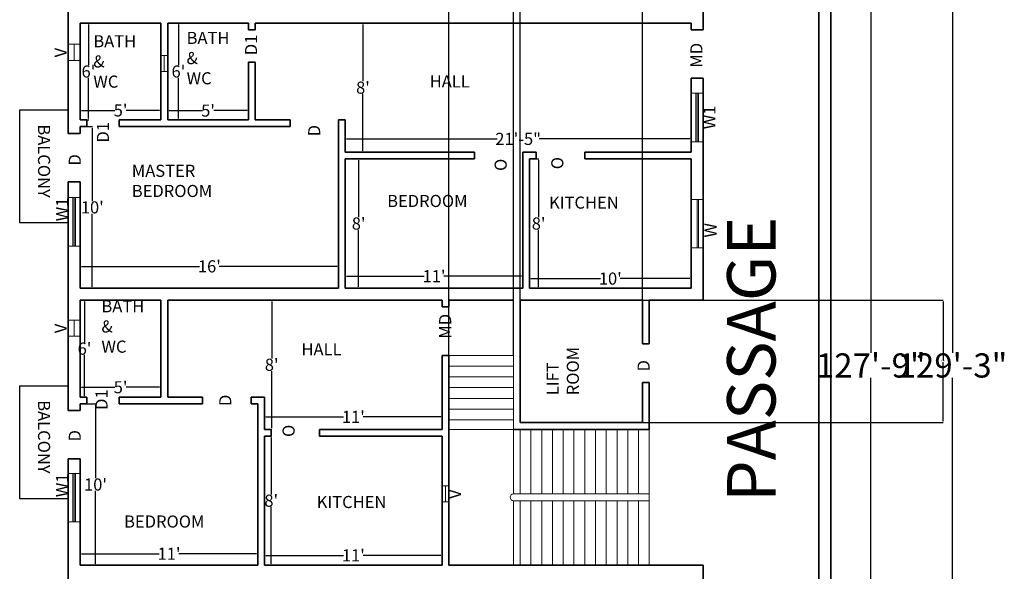
# Model space of a CAD drawing. Units: inches. Extents: x -2189 to 546, y 945 to 2684.
# Tile 3 of 10: x -866 to -134, y 1672 to 2082. Entities that reach past the tile are written whole.
import ezdxf

# ---------------------------------------------------------------- set-up
doc = ezdxf.new("R2010")
doc.units = ezdxf.units.IN
doc.header["$MEASUREMENT"] = 0
for name, color, linetype, lineweight in [('A-ANNO-DIMS', 2, 'Continuous', 13), ('A-ANNO-TEXT', 7, 'Continuous', 18), ('A-AREA-IDEN', 3, 'Continuous', 18), ('A-FLOR-BALC', 8, 'Continuous', 25), ('A-FLOR-STRS', 3, 'Continuous', 18), ('A-GLAZ', 4, 'Continuous', 18), ('A-WALL', 7, 'Continuous', 35)]:
    doc.layers.add(name, color=color, linetype=linetype, lineweight=lineweight)
doc.styles.get("Standard").update_dxf_attribs({"font": 'arial.ttf'})
doc.dimstyles.get("Standard").update_dxf_attribs({"dimtxt": 1, "dimasz": 1, "dimexe": 0.18, "dimexo": 0.0625, "dimgap": 0.09, "dimtad": 0, "dimtih": 1, "dimtoh": 1, "dimdec": 0, "dimzin": 0, "dimdsep": 46, "dimlunit": 3, "dimtxsty": 'Standard', "dimcen": 0.09, "dimadec": 0, "dimazin": 0, "dimtfac": 1, "dimtdec": 0, "dimtofl": 0, "dimtmove": 0, "dimatfit": 3, "dimfxl": 1, "dimtolj": 1, "dimtzin": 0, "dimarcsym": 0})

# ---------------------------------------------------------------- blocks, each defined once
blk = doc.blocks.new('*D37')
at = {"layer": 'A-ANNO-DIMS', "color": 0, "lineweight": -2, "transparency": 16777216}
for p, q in [((-820.78, 1676.24), (-820.78, 1684.89)), ((-819.78, 1684.71), (-762.08, 1684.71)), ((-689.78, 1684.71), (-747.48, 1684.71)), ((-688.78, 1676.24), (-688.78, 1684.89))]:
    blk.add_line(p, q, dxfattribs=at)
at = {"layer": 'A-ANNO-DIMS', "color": 0, "transparency": 16777216}
for points in [[(-819.78, 1684.88), (-819.78, 1684.54), (-820.78, 1684.71)], [(-689.78, 1684.88), (-689.78, 1684.54), (-688.78, 1684.71)]]:
    blk.add_solid(points, dxfattribs=at)
at = {"layer": 'Defpoints', "color": 0, "transparency": 16777216}
for p in [(-688.78, 1684.71), (-820.78, 1676.17), (-688.78, 1676.17)]:
    blk.add_point(p, dxfattribs=at)
at = {"layer": 'A-ANNO-DIMS', "color": 0, "transparency": 16777216, "insert": (-754.78, 1684.71), "char_height": 1, "attachment_point": 5}
blk.add_mtext("\\A1;{\\H9x;11'}", dxfattribs=at)
blk = doc.blocks.new('*D38')
at = {"layer": 'A-ANNO-DIMS', "color": 0, "lineweight": -2, "transparency": 16777216}
for p, q in [((-820.72, 1796.17), (-809.26, 1796.17)), ((-809.44, 1795.17), (-809.44, 1740.86)), ((-809.44, 1677.17), (-809.44, 1731.49)), ((-820.72, 1676.17), (-809.26, 1676.17))]:
    blk.add_line(p, q, dxfattribs=at)
at = {"layer": 'A-ANNO-DIMS', "color": 0, "transparency": 16777216}
for points in [[(-809.61, 1795.17), (-809.28, 1795.17), (-809.44, 1796.17)], [(-809.61, 1677.17), (-809.28, 1677.17), (-809.44, 1676.17)]]:
    blk.add_solid(points, dxfattribs=at)
at = {"layer": 'Defpoints', "color": 0, "transparency": 16777216}
for p in [(-820.78, 1796.17), (-809.44, 1796.17), (-820.78, 1676.17)]:
    blk.add_point(p, dxfattribs=at)
at = {"layer": 'A-ANNO-DIMS', "color": 0, "transparency": 16777216, "insert": (-809.44, 1736.17), "char_height": 1, "attachment_point": 5}
blk.add_mtext("\\A1;{\\H9x;10'}", dxfattribs=at)
blk = doc.blocks.new('*D39')
at = {"layer": 'A-ANNO-DIMS', "color": 0, "lineweight": -2, "transparency": 16777216}
for p, q in [((-820.78, 1801.24), (-820.78, 1808.68)), ((-819.78, 1808.5), (-795.01, 1808.5)), ((-761.78, 1808.5), (-786.55, 1808.5)), ((-760.78, 1801.24), (-760.78, 1808.68))]:
    blk.add_line(p, q, dxfattribs=at)
at = {"layer": 'A-ANNO-DIMS', "color": 0, "transparency": 16777216}
for points in [[(-819.78, 1808.66), (-819.78, 1808.33), (-820.78, 1808.5)], [(-761.78, 1808.66), (-761.78, 1808.33), (-760.78, 1808.5)]]:
    blk.add_solid(points, dxfattribs=at)
at = {"layer": 'Defpoints', "color": 0, "transparency": 16777216}
for p in [(-760.78, 1808.5), (-820.78, 1801.17), (-760.78, 1801.17)]:
    blk.add_point(p, dxfattribs=at)
at = {"layer": 'A-ANNO-DIMS', "color": 0, "transparency": 16777216, "insert": (-790.78, 1808.5), "char_height": 1, "attachment_point": 5}
blk.add_mtext("\\A1;{\\H9x;5'}", dxfattribs=at)
blk = doc.blocks.new('*D40')
at = {"layer": 'A-ANNO-DIMS', "color": 0, "lineweight": -2, "transparency": 16777216}
for p, q in [((-820.72, 1873.17), (-817.43, 1873.17)), ((-817.61, 1872.17), (-817.61, 1841.86)), ((-817.61, 1802.17), (-817.61, 1832.49)), ((-820.72, 1801.17), (-817.43, 1801.17))]:
    blk.add_line(p, q, dxfattribs=at)
at = {"layer": 'A-ANNO-DIMS', "color": 0, "transparency": 16777216}
for points in [[(-817.77, 1872.17), (-817.44, 1872.17), (-817.61, 1873.17)], [(-817.77, 1802.17), (-817.44, 1802.17), (-817.61, 1801.17)]]:
    blk.add_solid(points, dxfattribs=at)
at = {"layer": 'Defpoints', "color": 0, "transparency": 16777216}
for p in [(-820.78, 1873.17), (-817.61, 1873.17), (-820.78, 1801.17)]:
    blk.add_point(p, dxfattribs=at)
at = {"layer": 'A-ANNO-DIMS', "color": 0, "transparency": 16777216, "insert": (-817.61, 1837.17), "char_height": 1, "attachment_point": 5}
blk.add_mtext("\\A1;{\\H9x;6'}", dxfattribs=at)
blk = doc.blocks.new('*D41')
at = {"layer": 'A-ANNO-DIMS', "color": 0, "lineweight": -2, "transparency": 16777216}
for p, q in [((-683.78, 1676.24), (-683.78, 1683.7)), ((-682.78, 1683.52), (-625.08, 1683.52)), ((-552.78, 1683.52), (-610.48, 1683.52)), ((-551.78, 1676.24), (-551.78, 1683.7))]:
    blk.add_line(p, q, dxfattribs=at)
at = {"layer": 'A-ANNO-DIMS', "color": 0, "transparency": 16777216}
for points in [[(-682.78, 1683.68), (-682.78, 1683.35), (-683.78, 1683.52)], [(-552.78, 1683.68), (-552.78, 1683.35), (-551.78, 1683.52)]]:
    blk.add_solid(points, dxfattribs=at)
at = {"layer": 'Defpoints', "color": 0, "transparency": 16777216}
for p in [(-551.78, 1683.52), (-683.78, 1676.17), (-551.78, 1676.17)]:
    blk.add_point(p, dxfattribs=at)
at = {"layer": 'A-ANNO-DIMS', "color": 0, "transparency": 16777216, "insert": (-617.78, 1683.52), "char_height": 1, "attachment_point": 5}
blk.add_mtext("\\A1;{\\H9x;11'}", dxfattribs=at)
blk = doc.blocks.new('*D42')
at = {"layer": 'A-ANNO-DIMS', "color": 0, "lineweight": -2, "transparency": 16777216}
for p, q in [((-683.72, 1772.17), (-678.62, 1772.17)), ((-678.8, 1771.17), (-678.8, 1728.86)), ((-678.8, 1677.17), (-678.8, 1719.49)), ((-683.72, 1676.17), (-678.62, 1676.17))]:
    blk.add_line(p, q, dxfattribs=at)
at = {"layer": 'A-ANNO-DIMS', "color": 0, "transparency": 16777216}
for points in [[(-678.97, 1771.17), (-678.63, 1771.17), (-678.8, 1772.17)], [(-678.97, 1677.17), (-678.63, 1677.17), (-678.8, 1676.17)]]:
    blk.add_solid(points, dxfattribs=at)
at = {"layer": 'Defpoints', "color": 0, "transparency": 16777216}
for p in [(-683.78, 1772.17), (-683.78, 1676.17), (-678.8, 1676.17)]:
    blk.add_point(p, dxfattribs=at)
at = {"layer": 'A-ANNO-DIMS', "color": 0, "transparency": 16777216, "insert": (-678.8, 1724.17), "char_height": 1, "attachment_point": 5}
blk.add_mtext("\\A1;{\\H9x;8'}", dxfattribs=at)
blk = doc.blocks.new('*D43')
at = {"layer": 'A-ANNO-DIMS', "color": 0, "lineweight": -2, "transparency": 16777216}
for p, q in [((-683.72, 1873.17), (-678.29, 1873.17)), ((-678.47, 1872.17), (-678.47, 1829.86)), ((-678.47, 1778.17), (-678.47, 1820.49)), ((-683.72, 1777.17), (-678.29, 1777.17))]:
    blk.add_line(p, q, dxfattribs=at)
at = {"layer": 'A-ANNO-DIMS', "color": 0, "transparency": 16777216}
for points in [[(-678.64, 1872.17), (-678.31, 1872.17), (-678.47, 1873.17)], [(-678.64, 1778.17), (-678.31, 1778.17), (-678.47, 1777.17)]]:
    blk.add_solid(points, dxfattribs=at)
at = {"layer": 'Defpoints', "color": 0, "transparency": 16777216}
for p in [(-683.78, 1873.17), (-678.47, 1873.17), (-683.78, 1777.17)]:
    blk.add_point(p, dxfattribs=at)
at = {"layer": 'A-ANNO-DIMS', "color": 0, "transparency": 16777216, "insert": (-678.47, 1825.17), "char_height": 1, "attachment_point": 5}
blk.add_mtext("\\A1;{\\H9x;8'}", dxfattribs=at)
blk = doc.blocks.new('*D44')
at = {"layer": 'A-ANNO-DIMS', "color": 0, "lineweight": -2, "transparency": 16777216}
for p, q in [((-683.78, 1777.24), (-683.78, 1786.65)), ((-682.78, 1786.47), (-625.08, 1786.47)), ((-552.78, 1786.47), (-610.48, 1786.47)), ((-551.78, 1777.24), (-551.78, 1786.65))]:
    blk.add_line(p, q, dxfattribs=at)
at = {"layer": 'A-ANNO-DIMS', "color": 0, "transparency": 16777216}
for points in [[(-682.78, 1786.64), (-682.78, 1786.31), (-683.78, 1786.47)], [(-552.78, 1786.64), (-552.78, 1786.31), (-551.78, 1786.47)]]:
    blk.add_solid(points, dxfattribs=at)
at = {"layer": 'Defpoints', "color": 0, "transparency": 16777216}
for p in [(-551.78, 1786.47), (-683.78, 1777.17), (-551.78, 1777.17)]:
    blk.add_point(p, dxfattribs=at)
at = {"layer": 'A-ANNO-DIMS', "color": 0, "transparency": 16777216, "insert": (-617.78, 1786.47), "char_height": 1, "attachment_point": 5}
blk.add_mtext("\\A1;{\\H9x;11'}", dxfattribs=at)
blk = doc.blocks.new('*D45')
at = {"layer": 'A-ANNO-DIMS', "color": 0, "lineweight": -2, "transparency": 16777216}
for p, q in [((-820.78, 1882.24), (-820.78, 1898.51)), ((-819.78, 1898.33), (-732.08, 1898.33)), ((-629.78, 1898.33), (-717.48, 1898.33)), ((-628.78, 1882.24), (-628.78, 1898.51))]:
    blk.add_line(p, q, dxfattribs=at)
at = {"layer": 'A-ANNO-DIMS', "color": 0, "transparency": 16777216}
for points in [[(-819.78, 1898.5), (-819.78, 1898.16), (-820.78, 1898.33)], [(-629.78, 1898.5), (-629.78, 1898.16), (-628.78, 1898.33)]]:
    blk.add_solid(points, dxfattribs=at)
at = {"layer": 'Defpoints', "color": 0, "transparency": 16777216}
for p in [(-628.78, 1898.33), (-820.78, 1882.17), (-628.78, 1882.17)]:
    blk.add_point(p, dxfattribs=at)
at = {"layer": 'A-ANNO-DIMS', "color": 0, "transparency": 16777216, "insert": (-724.78, 1898.33), "char_height": 1, "attachment_point": 5}
blk.add_mtext("\\A1;{\\H9x;16'}", dxfattribs=at)
blk = doc.blocks.new('*D46')
at = {"layer": 'A-ANNO-DIMS', "color": 0, "lineweight": -2, "transparency": 16777216}
for p, q in [((-820.72, 2002.17), (-811.63, 2002.17)), ((-811.81, 2001.17), (-811.81, 1946.86)), ((-811.81, 1883.17), (-811.81, 1937.49)), ((-820.72, 1882.17), (-811.63, 1882.17))]:
    blk.add_line(p, q, dxfattribs=at)
at = {"layer": 'A-ANNO-DIMS', "color": 0, "transparency": 16777216}
for points in [[(-811.98, 2001.17), (-811.65, 2001.17), (-811.81, 2002.17)], [(-811.98, 1883.17), (-811.65, 1883.17), (-811.81, 1882.17)]]:
    blk.add_solid(points, dxfattribs=at)
at = {"layer": 'Defpoints', "color": 0, "transparency": 16777216}
for p in [(-820.78, 2002.17), (-820.78, 1882.17), (-811.81, 1882.17)]:
    blk.add_point(p, dxfattribs=at)
at = {"layer": 'A-ANNO-DIMS', "color": 0, "transparency": 16777216, "insert": (-811.81, 1942.17), "char_height": 1, "attachment_point": 5}
blk.add_mtext("\\A1;{\\H9x;10'}", dxfattribs=at)
blk = doc.blocks.new('*D47')
at = {"layer": 'A-ANNO-DIMS', "color": 0, "lineweight": -2, "transparency": 16777216}
for p, q in [((-820.78, 2007.24), (-820.78, 2014.43)), ((-819.78, 2014.25), (-795.01, 2014.25)), ((-761.78, 2014.25), (-786.55, 2014.25)), ((-760.78, 2007.24), (-760.78, 2014.43))]:
    blk.add_line(p, q, dxfattribs=at)
at = {"layer": 'A-ANNO-DIMS', "color": 0, "transparency": 16777216}
for points in [[(-819.78, 2014.42), (-819.78, 2014.08), (-820.78, 2014.25)], [(-761.78, 2014.42), (-761.78, 2014.08), (-760.78, 2014.25)]]:
    blk.add_solid(points, dxfattribs=at)
at = {"layer": 'Defpoints', "color": 0, "transparency": 16777216}
for p in [(-760.78, 2014.25), (-820.78, 2007.17), (-760.78, 2007.17)]:
    blk.add_point(p, dxfattribs=at)
at = {"layer": 'A-ANNO-DIMS', "color": 0, "transparency": 16777216, "insert": (-790.78, 2014.25), "char_height": 1, "attachment_point": 5}
blk.add_mtext("\\A1;{\\H9x;5'}", dxfattribs=at)
blk = doc.blocks.new('*D48')
at = {"layer": 'A-ANNO-DIMS', "color": 0, "lineweight": -2, "transparency": 16777216}
for p, q in [((-820.72, 2079.17), (-814.5, 2079.17)), ((-814.68, 2078.17), (-814.68, 2047.86)), ((-814.68, 2008.17), (-814.68, 2038.49)), ((-820.72, 2007.17), (-814.5, 2007.17))]:
    blk.add_line(p, q, dxfattribs=at)
at = {"layer": 'A-ANNO-DIMS', "color": 0, "transparency": 16777216}
for points in [[(-814.84, 2078.17), (-814.51, 2078.17), (-814.68, 2079.17)], [(-814.84, 2008.17), (-814.51, 2008.17), (-814.68, 2007.17)]]:
    blk.add_solid(points, dxfattribs=at)
at = {"layer": 'Defpoints', "color": 0, "transparency": 16777216}
for p in [(-820.78, 2079.17), (-814.68, 2079.17), (-820.78, 2007.17)]:
    blk.add_point(p, dxfattribs=at)
at = {"layer": 'A-ANNO-DIMS', "color": 0, "transparency": 16777216, "insert": (-814.68, 2043.17), "char_height": 1, "attachment_point": 5}
blk.add_mtext("\\A1;{\\H9x;6'}", dxfattribs=at)
blk = doc.blocks.new('*D49')
at = {"layer": 'A-ANNO-DIMS', "color": 0, "lineweight": -2, "transparency": 16777216}
for p, q in [((-755.78, 2007.24), (-755.78, 2014.31)), ((-754.78, 2014.13), (-730.01, 2014.13)), ((-696.78, 2014.13), (-721.55, 2014.13)), ((-695.78, 2007.24), (-695.78, 2014.31))]:
    blk.add_line(p, q, dxfattribs=at)
at = {"layer": 'A-ANNO-DIMS', "color": 0, "transparency": 16777216}
for points in [[(-754.78, 2014.3), (-754.78, 2013.96), (-755.78, 2014.13)], [(-696.78, 2014.3), (-696.78, 2013.96), (-695.78, 2014.13)]]:
    blk.add_solid(points, dxfattribs=at)
at = {"layer": 'Defpoints', "color": 0, "transparency": 16777216}
for p in [(-755.78, 2014.13), (-755.78, 2007.17), (-695.78, 2007.17)]:
    blk.add_point(p, dxfattribs=at)
at = {"layer": 'A-ANNO-DIMS', "color": 0, "transparency": 16777216, "insert": (-725.78, 2014.13), "char_height": 1, "attachment_point": 5}
blk.add_mtext("\\A1;{\\H9x;5'}", dxfattribs=at)
blk = doc.blocks.new('*D50')
at = {"layer": 'A-ANNO-DIMS', "color": 0, "lineweight": -2, "transparency": 16777216}
for p, q in [((-755.72, 2079.17), (-747.61, 2079.17)), ((-747.79, 2078.17), (-747.79, 2047.86)), ((-747.79, 2008.17), (-747.79, 2038.49)), ((-755.72, 2007.17), (-747.61, 2007.17))]:
    blk.add_line(p, q, dxfattribs=at)
at = {"layer": 'A-ANNO-DIMS', "color": 0, "transparency": 16777216}
for points in [[(-747.95, 2078.17), (-747.62, 2078.17), (-747.79, 2079.17)], [(-747.95, 2008.17), (-747.62, 2008.17), (-747.79, 2007.17)]]:
    blk.add_solid(points, dxfattribs=at)
at = {"layer": 'Defpoints', "color": 0, "transparency": 16777216}
for p in [(-755.78, 2079.17), (-747.79, 2079.17), (-755.78, 2007.17)]:
    blk.add_point(p, dxfattribs=at)
at = {"layer": 'A-ANNO-DIMS', "color": 0, "transparency": 16777216, "insert": (-747.79, 2043.17), "char_height": 1, "attachment_point": 5}
blk.add_mtext("\\A1;{\\H9x;6'}", dxfattribs=at)
blk = doc.blocks.new('*D51')
at = {"layer": 'A-ANNO-DIMS', "color": 0, "lineweight": -2, "transparency": 16777216}
for p, q in [((-623.78, 1882.24), (-623.78, 1891.19)), ((-622.78, 1891.01), (-565.08, 1891.01)), ((-492.78, 1891.01), (-550.48, 1891.01)), ((-491.78, 1882.24), (-491.78, 1891.19))]:
    blk.add_line(p, q, dxfattribs=at)
at = {"layer": 'A-ANNO-DIMS', "color": 0, "transparency": 16777216}
for points in [[(-622.78, 1891.17), (-622.78, 1890.84), (-623.78, 1891.01)], [(-492.78, 1891.17), (-492.78, 1890.84), (-491.78, 1891.01)]]:
    blk.add_solid(points, dxfattribs=at)
at = {"layer": 'Defpoints', "color": 0, "transparency": 16777216}
for p in [(-623.78, 1891.01), (-623.78, 1882.17), (-491.78, 1882.17)]:
    blk.add_point(p, dxfattribs=at)
at = {"layer": 'A-ANNO-DIMS', "color": 0, "transparency": 16777216, "insert": (-557.78, 1891.01), "char_height": 1, "attachment_point": 5}
blk.add_mtext("\\A1;{\\H9x;11'}", dxfattribs=at)
blk = doc.blocks.new('*D52')
at = {"layer": 'A-ANNO-DIMS', "color": 0, "lineweight": -2, "transparency": 16777216}
for p, q in [((-623.72, 1978.17), (-613.65, 1978.17)), ((-613.83, 1977.17), (-613.83, 1934.86)), ((-613.83, 1883.17), (-613.83, 1925.49)), ((-623.72, 1882.17), (-613.65, 1882.17))]:
    blk.add_line(p, q, dxfattribs=at)
at = {"layer": 'A-ANNO-DIMS', "color": 0, "transparency": 16777216}
for points in [[(-613.99, 1977.17), (-613.66, 1977.17), (-613.83, 1978.17)], [(-613.99, 1883.17), (-613.66, 1883.17), (-613.83, 1882.17)]]:
    blk.add_solid(points, dxfattribs=at)
at = {"layer": 'Defpoints', "color": 0, "transparency": 16777216}
for p in [(-623.78, 1978.17), (-613.83, 1978.17), (-623.78, 1882.17)]:
    blk.add_point(p, dxfattribs=at)
at = {"layer": 'A-ANNO-DIMS', "color": 0, "transparency": 16777216, "insert": (-613.83, 1930.17), "char_height": 1, "attachment_point": 5}
blk.add_mtext("\\A1;{\\H9x;8'}", dxfattribs=at)
blk = doc.blocks.new('*D53')
at = {"layer": 'A-ANNO-DIMS', "color": 0, "lineweight": -2, "transparency": 16777216}
for p, q in [((-486.72, 1978.17), (-479.88, 1978.17)), ((-480.06, 1977.17), (-480.06, 1934.86)), ((-480.06, 1883.17), (-480.06, 1925.49)), ((-486.72, 1882.17), (-479.88, 1882.17))]:
    blk.add_line(p, q, dxfattribs=at)
at = {"layer": 'A-ANNO-DIMS', "color": 0, "transparency": 16777216}
for points in [[(-480.23, 1977.17), (-479.9, 1977.17), (-480.06, 1978.17)], [(-480.23, 1883.17), (-479.9, 1883.17), (-480.06, 1882.17)]]:
    blk.add_solid(points, dxfattribs=at)
at = {"layer": 'Defpoints', "color": 0, "transparency": 16777216}
for p in [(-486.78, 1978.17), (-480.06, 1978.17), (-486.78, 1882.17)]:
    blk.add_point(p, dxfattribs=at)
at = {"layer": 'A-ANNO-DIMS', "color": 0, "transparency": 16777216, "insert": (-480.06, 1930.17), "char_height": 1, "attachment_point": 5}
blk.add_mtext("\\A1;{\\H9x;8'}", dxfattribs=at)
blk = doc.blocks.new('*D54')
at = {"layer": 'A-ANNO-DIMS', "color": 0, "lineweight": -2, "transparency": 16777216}
for p, q in [((-486.78, 1882.24), (-486.78, 1889.42)), ((-485.78, 1889.24), (-434.08, 1889.24)), ((-367.78, 1889.24), (-419.48, 1889.24)), ((-366.78, 1882.24), (-366.78, 1889.42))]:
    blk.add_line(p, q, dxfattribs=at)
at = {"layer": 'A-ANNO-DIMS', "color": 0, "transparency": 16777216}
for points in [[(-485.78, 1889.4), (-485.78, 1889.07), (-486.78, 1889.24)], [(-367.78, 1889.4), (-367.78, 1889.07), (-366.78, 1889.24)]]:
    blk.add_solid(points, dxfattribs=at)
at = {"layer": 'Defpoints', "color": 0, "transparency": 16777216}
for p in [(-486.78, 1889.24), (-486.78, 1882.17), (-366.78, 1882.17)]:
    blk.add_point(p, dxfattribs=at)
at = {"layer": 'A-ANNO-DIMS', "color": 0, "transparency": 16777216, "insert": (-426.78, 1889.24), "char_height": 1, "attachment_point": 5}
blk.add_mtext("\\A1;{\\H9x;10'}", dxfattribs=at)
blk = doc.blocks.new('*D55')
at = {"layer": 'A-ANNO-DIMS', "color": 0, "lineweight": -2, "transparency": 16777216}
for p, q in [((-623.72, 2079.17), (-610.46, 2079.17)), ((-610.64, 2078.17), (-610.64, 2035.86)), ((-610.64, 1984.17), (-610.64, 2026.49)), ((-623.72, 1983.17), (-610.46, 1983.17))]:
    blk.add_line(p, q, dxfattribs=at)
at = {"layer": 'A-ANNO-DIMS', "color": 0, "transparency": 16777216}
for points in [[(-610.81, 2078.17), (-610.48, 2078.17), (-610.64, 2079.17)], [(-610.81, 1984.17), (-610.48, 1984.17), (-610.64, 1983.17)]]:
    blk.add_solid(points, dxfattribs=at)
at = {"layer": 'Defpoints', "color": 0, "transparency": 16777216}
for p in [(-623.78, 2079.17), (-610.64, 2079.17), (-623.78, 1983.17)]:
    blk.add_point(p, dxfattribs=at)
at = {"layer": 'A-ANNO-DIMS', "color": 0, "transparency": 16777216, "insert": (-610.64, 2031.17), "char_height": 1, "attachment_point": 5}
blk.add_mtext("\\A1;{\\H9x;8'}", dxfattribs=at)
blk = doc.blocks.new('*D56')
at = {"layer": 'A-ANNO-DIMS', "color": 0, "lineweight": -2, "transparency": 16777216}
for p, q in [((-623.78, 1983.24), (-623.78, 1993.26)), ((-622.78, 1993.08), (-510.9, 1993.08)), ((-367.78, 1993.08), (-479.65, 1993.08)), ((-366.78, 1983.24), (-366.78, 1993.26))]:
    blk.add_line(p, q, dxfattribs=at)
at = {"layer": 'A-ANNO-DIMS', "color": 0, "transparency": 16777216}
for points in [[(-622.78, 1993.24), (-622.78, 1992.91), (-623.78, 1993.08)], [(-367.78, 1993.24), (-367.78, 1992.91), (-366.78, 1993.08)]]:
    blk.add_solid(points, dxfattribs=at)
at = {"layer": 'Defpoints', "color": 0, "transparency": 16777216}
for p in [(-623.78, 1993.08), (-623.78, 1983.17), (-366.78, 1983.17)]:
    blk.add_point(p, dxfattribs=at)
at = {"layer": 'A-ANNO-DIMS', "color": 0, "transparency": 16777216, "insert": (-495.28, 1993.08), "char_height": 1, "attachment_point": 5}
blk.add_mtext('\\A1;{\\H9x;21\'-5"}', dxfattribs=at)
blk = doc.blocks.new('*D79')
at = {"layer": 'A-ANNO-DIMS', "color": 0, "lineweight": -2, "transparency": 16777216}
for p, q in [((-262.72, 2600.17), (-172.26, 2600.17)), ((-172.44, 2599.17), (-172.44, 1833.96)), ((-172.44, 1050.17), (-172.44, 1815.39)), ((-262.72, 1049.17), (-172.26, 1049.17))]:
    blk.add_line(p, q, dxfattribs=at)
at = {"layer": 'A-ANNO-DIMS', "color": 0, "transparency": 16777216}
for points in [[(-172.6, 2599.17), (-172.27, 2599.17), (-172.44, 2600.17)], [(-172.6, 1050.17), (-172.27, 1050.17), (-172.44, 1049.17)]]:
    blk.add_solid(points, dxfattribs=at)
at = {"layer": 'Defpoints', "color": 0, "transparency": 16777216}
for p in [(-262.78, 2600.17), (-172.44, 2600.17), (-262.78, 1049.17)]:
    blk.add_point(p, dxfattribs=at)
at = {"layer": 'A-ANNO-DIMS', "color": 0, "transparency": 16777216, "insert": (-172.44, 1824.67), "char_height": 1, "attachment_point": 5}
blk.add_mtext('\\A1;{\\H18x;129\'-3"}', dxfattribs=at)
blk = doc.blocks.new('*D80')
at = {"layer": 'A-ANNO-DIMS', "color": 0, "lineweight": -2, "transparency": 16777216}
for p, q in [((-271.72, 2591.17), (-233.01, 2591.17)), ((-233.19, 2590.17), (-233.19, 1833.95)), ((-233.19, 1059.17), (-233.19, 1815.39)), ((-271.72, 1058.17), (-233.01, 1058.17))]:
    blk.add_line(p, q, dxfattribs=at)
at = {"layer": 'A-ANNO-DIMS', "color": 0, "transparency": 16777216}
for points in [[(-233.36, 2590.17), (-233.03, 2590.17), (-233.19, 2591.17)], [(-233.36, 1059.17), (-233.03, 1059.17), (-233.19, 1058.17)]]:
    blk.add_solid(points, dxfattribs=at)
at = {"layer": 'Defpoints', "color": 0, "transparency": 16777216}
for p in [(-271.78, 2591.17), (-233.19, 2591.17), (-271.78, 1058.17)]:
    blk.add_point(p, dxfattribs=at)
at = {"layer": 'A-ANNO-DIMS', "color": 0, "transparency": 16777216, "insert": (-233.19, 1824.67), "char_height": 1, "attachment_point": 5}
blk.add_mtext('\\A1;{\\H18x;127\'-9"}', dxfattribs=at)
blk = doc.blocks.new('WIN-36X9')
for p, q in [((0, 5.5), (36, 5.5)), ((0, 5.5), (36, 5.5)), ((0, 4.5), (36, 4.5)), ((0, 3.5), (36, 3.5))]:
    blk.add_line(p, q)
blk.add_lwpolyline([(0, 0), (0, 9), (36, 9), (36, 0)], close=True)
blk = doc.blocks.new('VENT-12X5')
blk.add_line((2.5, 12), (2.5, 0))
blk.add_lwpolyline([(5, 12), (0, 12), (0, 0), (5, 0)], close=True)
blk = doc.blocks.new('WIN-36X9-TWINLINE')
for p, q in [((4.5, 0), (4.5, 36)), ((5.5, 0), (5.5, 36))]:
    blk.add_line(p, q)
blk.add_lwpolyline([(9, 0), (0, 0), (0, 36), (9, 36)], close=True)
blk = doc.blocks.new('VENT-12X9-SINGLELINE')
blk.add_line((4.5, 12), (4.5, 0))
blk.add_lwpolyline([(0, 12), (9, 12), (9, 0), (0, 0)], close=True)
blk = doc.blocks.new('BALCONY-36X84')
for p, q in [((0, 0), (0, 84)), ((0, 84), (36, 84)), ((36, 0), (0, 0))]:
    blk.add_line(p, q)
blk = doc.blocks.new('*D104')
at = {"layer": 'A-ANNO-DIMS', "color": 0, "lineweight": -2, "transparency": 16777216}
for p, q in [((-493.78, 1873.24), (-493.78, 2683.65)), ((-492.78, 2683.47), (-449.69, 2683.47)), ((-403.78, 2683.47), (-446.86, 2683.47)), ((-402.78, 1873.24), (-402.78, 2683.65))]:
    blk.add_line(p, q, dxfattribs=at)
at = {"layer": 'A-ANNO-DIMS', "color": 0, "transparency": 16777216}
for points in [[(-492.78, 2683.64), (-492.78, 2683.31), (-493.78, 2683.47)], [(-403.78, 2683.64), (-403.78, 2683.31), (-402.78, 2683.47)]]:
    blk.add_solid(points, dxfattribs=at)
at = {"layer": 'Defpoints', "color": 0, "transparency": 16777216}
for p in [(-402.78, 2683.47), (-493.78, 1873.17), (-402.78, 1873.17)]:
    blk.add_point(p, dxfattribs=at)
at = {"layer": 'A-ANNO-DIMS', "color": 0, "transparency": 16777216, "insert": (-448.28, 2683.47), "char_height": 1, "attachment_point": 5}
blk.add_mtext('\\A1;7\'-7"', dxfattribs=at)
blk = doc.blocks.new('*D105')
at = {"layer": 'A-ANNO-DIMS', "color": 0, "lineweight": -2, "transparency": 16777216}
for p, q in [((-402.72, 1873.17), (-179.3, 1873.17)), ((-179.48, 1872.17), (-179.48, 1828.26)), ((-179.48, 1783.17), (-179.48, 1827.08)), ((-402.72, 1782.17), (-179.3, 1782.17))]:
    blk.add_line(p, q, dxfattribs=at)
at = {"layer": 'A-ANNO-DIMS', "color": 0, "transparency": 16777216}
for points in [[(-179.65, 1872.17), (-179.31, 1872.17), (-179.48, 1873.17)], [(-179.65, 1783.17), (-179.31, 1783.17), (-179.48, 1782.17)]]:
    blk.add_solid(points, dxfattribs=at)
at = {"layer": 'Defpoints', "color": 0, "transparency": 16777216}
for p in [(-402.78, 1873.17), (-179.48, 1873.17), (-402.78, 1782.17)]:
    blk.add_point(p, dxfattribs=at)
at = {"layer": 'A-ANNO-DIMS', "color": 0, "transparency": 16777216, "insert": (-179.48, 1827.67), "char_height": 1, "attachment_point": 5}
blk.add_mtext('\\A1;7\'-7"', dxfattribs=at)
blk = doc.blocks.new('*D106')
at = {"layer": 'A-ANNO-DIMS', "color": 0, "lineweight": -2, "transparency": 16777216}
for p, q in [((-546.78, 1832.24), (-546.78, 2683.65)), ((-545.78, 2683.47), (-524.22, 2683.47)), ((-499.78, 2683.47), (-521.34, 2683.47)), ((-498.78, 1832.24), (-498.78, 2683.65))]:
    blk.add_line(p, q, dxfattribs=at)
at = {"layer": 'A-ANNO-DIMS', "color": 0, "transparency": 16777216}
for points in [[(-545.78, 2683.64), (-545.78, 2683.31), (-546.78, 2683.47)], [(-499.78, 2683.64), (-499.78, 2683.31), (-498.78, 2683.47)]]:
    blk.add_solid(points, dxfattribs=at)
at = {"layer": 'Defpoints', "color": 0, "transparency": 16777216}
for p in [(-498.78, 2683.47), (-546.78, 1832.17), (-498.78, 1832.17)]:
    blk.add_point(p, dxfattribs=at)
at = {"layer": 'A-ANNO-DIMS', "color": 0, "transparency": 16777216, "insert": (-522.78, 2683.47), "char_height": 1, "attachment_point": 5}
blk.add_mtext('\\A1;4\'-0"', dxfattribs=at)

msp = doc.modelspace()

# ---------------------------------------------------------------- linework, layer by layer
at = {"layer": 'A-FLOR-STRS'}
for p, q in [((-498.78, 1729.17), (-498.78, 1873.17)), ((-546.78, 1832.17), (-498.78, 1832.17)), ((-546.78, 1824.17), (-498.78, 1824.17)), ((-546.78, 1816.17), (-498.78, 1816.17)), ((-546.78, 1808.17), (-498.78, 1808.17)), ((-546.78, 1800.17), (-498.78, 1800.17)), ((-546.78, 1792.17), (-498.78, 1792.17)), ((-546.78, 1792.17), (-498.78, 1792.17)), ((-546.78, 1784.17), (-498.78, 1784.17)), ((-546.78, 1777.17), (-498.78, 1777.17)), ((-493.78, 1729.17), (-493.78, 1777.16)), ((-485.78, 1729.17), (-485.78, 1777.16)), ((-477.78, 1729.17), (-477.78, 1777.16)), ((-469.78, 1729.17), (-469.78, 1777.16)), ((-461.78, 1729.17), (-461.78, 1777.16)), ((-453.78, 1729.17), (-453.78, 1777.16)), ((-445.78, 1729.17), (-445.78, 1777.16)), ((-437.78, 1729.17), (-437.78, 1777.16)), ((-429.78, 1729.17), (-429.78, 1777.16)), ((-421.78, 1729.17), (-421.78, 1777.16)), ((-413.78, 1729.17), (-413.78, 1777.16)), ((-405.78, 1729.17), (-405.78, 1777.16)), ((-397.78, 1676.17), (-397.78, 1777.16)), ((-397.78, 1729.17), (-498.78, 1729.17)), ((-498.78, 1676.17), (-498.78, 1724.17)), ((-397.78, 1724.17), (-498.78, 1724.17)), ((-493.78, 1676.17), (-493.78, 1724.17)), ((-485.78, 1676.17), (-485.78, 1724.17)), ((-477.78, 1676.17), (-477.78, 1724.17)), ((-469.78, 1676.17), (-469.78, 1724.17)), ((-461.78, 1676.17), (-461.78, 1724.17)), ((-453.78, 1676.17), (-453.78, 1724.17)), ((-445.78, 1676.17), (-445.78, 1724.17)), ((-437.78, 1676.17), (-437.78, 1724.17)), ((-429.78, 1676.17), (-429.78, 1724.17)), ((-421.78, 1676.17), (-421.78, 1724.17)), ((-413.78, 1676.17), (-413.78, 1724.17)), ((-405.78, 1676.17), (-405.78, 1724.17))]:
    msp.add_line(p, q, dxfattribs=at)
msp.add_arc((-498.78, 1726.67), 2.5, 90, 270, dxfattribs=at)
at = {"layer": 'A-WALL'}
for p, q in [((-262.78, 2600.17), (-262.78, 1049.17)), ((-271.78, 2591.17), (-271.78, 1058.17)), ((-357.78, 2074.17), (-357.78, 2240.2)), ((-829.78, 1997.17), (-829.78, 2163.17)), ((-820.78, 2007.17), (-820.78, 2079.17)), ((-760.78, 2079.17), (-820.78, 2079.17)), ((-760.78, 2007.17), (-760.78, 2079.17)), ((-755.78, 2007.17), (-755.78, 2079.17)), ((-695.78, 2079.17), (-755.78, 2079.17)), ((-695.78, 2074.17), (-695.78, 2079.17)), ((-366.78, 2079.17), (-690.78, 2079.17)), ((-690.78, 2074.17), (-690.78, 2079.17)), ((-366.78, 2074.17), (-366.78, 2079.17)), ((-695.78, 2074.17), (-690.78, 2074.17)), ((-366.78, 2074.17), (-357.78, 2074.17)), ((-695.78, 2007.17), (-695.78, 2050.17)), ((-695.78, 2050.17), (-690.78, 2050.17)), ((-690.78, 2007.17), (-690.78, 2050.17)), ((-366.78, 1983.17), (-366.78, 2038.17)), ((-366.78, 2038.17), (-357.78, 2038.17)), ((-357.78, 1873.17), (-357.78, 2038.17)), ((-815.78, 2007.17), (-820.78, 2007.17)), ((-815.78, 2007.17), (-815.78, 2002.17)), ((-760.78, 2007.17), (-791.78, 2007.17)), ((-791.78, 2007.17), (-791.78, 2002.17)), ((-695.78, 2007.17), (-755.78, 2007.17)), ((-664.78, 2007.17), (-690.78, 2007.17)), ((-664.78, 2002.17), (-664.78, 2007.17)), ((-628.78, 1882.17), (-628.78, 2007.17)), ((-623.78, 2007.17), (-628.78, 2007.17)), ((-623.78, 1983.17), (-623.78, 2007.17)), ((-820.78, 1997.17), (-820.78, 2002.17)), ((-815.78, 2002.17), (-820.78, 2002.17)), ((-664.78, 2002.17), (-791.78, 2002.17)), ((-820.78, 1997.17), (-829.78, 1997.17)), ((-527.78, 1983.17), (-623.78, 1983.17)), ((-623.78, 1882.17), (-623.78, 1978.17)), ((-527.78, 1978.17), (-623.78, 1978.17)), ((-527.78, 1983.17), (-527.78, 1978.17)), ((-491.78, 1983.17), (-486.78, 1983.17)), ((-491.78, 1983.17), (-491.78, 1978.17)), ((-491.78, 1882.17), (-491.78, 1978.17)), ((-481.78, 1983.17), (-486.78, 1983.17)), ((-486.78, 1882.17), (-486.78, 1978.17)), ((-481.78, 1978.17), (-486.78, 1978.17)), ((-481.78, 1983.17), (-481.78, 1978.17)), ((-366.78, 1983.17), (-445.78, 1983.17)), ((-445.78, 1983.17), (-445.78, 1978.17)), ((-366.78, 1978.17), (-445.78, 1978.17)), ((-366.78, 1882.17), (-366.78, 1978.17)), ((-829.78, 1791.17), (-829.78, 1961.17)), ((-820.78, 1961.17), (-829.78, 1961.17)), ((-820.78, 1882.17), (-820.78, 1961.17)), ((-628.78, 1882.17), (-820.78, 1882.17)), ((-491.78, 1882.17), (-623.78, 1882.17)), ((-366.78, 1882.17), (-486.78, 1882.17)), ((-820.78, 1801.17), (-820.78, 1873.17)), ((-760.78, 1873.17), (-820.78, 1873.17)), ((-760.78, 1801.17), (-760.78, 1873.17)), ((-755.78, 1801.17), (-755.78, 1873.17)), ((-551.78, 1873.17), (-755.78, 1873.17)), ((-551.78, 1868.17), (-551.78, 1873.17)), ((-551.78, 1868.17), (-546.78, 1868.17)), ((-546.78, 1868.17), (-546.78, 1873.17)), ((-498.78, 1873.17), (-546.78, 1873.17)), ((-493.78, 1782.17), (-493.78, 1873.17)), ((-402.78, 1873.17), (-493.78, 1873.17)), ((-402.78, 1840.74), (-402.78, 1873.17)), ((-357.78, 1873.17), (-397.78, 1873.17)), ((-397.78, 1840.74), (-397.78, 1873.17)), ((-402.78, 1840.74), (-397.78, 1840.74)), ((-551.78, 1777.17), (-551.78, 1832.17)), ((-551.78, 1832.17), (-546.78, 1832.17)), ((-546.78, 1777.17), (-546.78, 1832.17)), ((-402.78, 1782.17), (-402.78, 1811.96)), ((-402.78, 1811.96), (-397.78, 1811.96)), ((-397.78, 1777.16), (-397.78, 1811.96)), ((-815.78, 1801.17), (-820.78, 1801.17)), ((-815.78, 1801.17), (-815.78, 1796.17)), ((-760.78, 1801.17), (-791.78, 1801.17)), ((-791.78, 1801.17), (-791.78, 1796.17)), ((-729.78, 1801.17), (-755.78, 1801.17)), ((-729.78, 1801.17), (-729.78, 1796.17)), ((-683.78, 1801.17), (-693.78, 1801.17)), ((-693.78, 1801.17), (-693.78, 1796.17)), ((-683.78, 1777.17), (-683.78, 1801.17)), ((-820.78, 1791.17), (-820.78, 1796.17)), ((-815.78, 1796.17), (-820.78, 1796.17)), ((-729.78, 1796.17), (-791.78, 1796.17)), ((-688.78, 1796.17), (-693.78, 1796.17)), ((-688.78, 1676.17), (-688.78, 1796.17)), ((-820.78, 1791.17), (-829.78, 1791.17)), ((-402.78, 1782.17), (-493.78, 1782.17)), ((-678.78, 1777.17), (-683.78, 1777.17)), ((-683.78, 1676.17), (-683.78, 1772.17)), ((-678.78, 1772.17), (-683.78, 1772.17)), ((-678.78, 1772.17), (-678.78, 1777.17)), ((-551.78, 1777.17), (-642.84, 1777.17)), ((-642.84, 1772.17), (-642.84, 1777.17)), ((-551.78, 1772.17), (-642.84, 1772.17)), ((-551.78, 1676.17), (-551.78, 1772.17)), ((-546.78, 1772.17), (-546.78, 1777.17)), ((-546.78, 1676.17), (-546.78, 1772.17)), ((-397.78, 1777.17), (-498.78, 1777.17)), ((-829.78, 1585.17), (-829.78, 1755.17)), ((-820.78, 1755.17), (-829.78, 1755.17)), ((-820.78, 1676.17), (-820.78, 1755.17)), ((-688.78, 1676.17), (-820.78, 1676.17)), ((-551.78, 1676.17), (-683.78, 1676.17)), ((-357.78, 1676.17), (-546.78, 1676.17)), ((-357.78, 1662.17), (-357.78, 1676.17))]:
    msp.add_line(p, q, dxfattribs=at)

# ---------------------------------------------------------------- block references
at = {"layer": 'A-FLOR-BALC'}
for p in [(-865.78, 1930.66), (-865.78, 1725.62)]:
    msp.add_blockref('BALCONY-36X84', p, dxfattribs=at)
at = {"layer": 'A-GLAZ'}
for name, p in [('VENT-12X9-SINGLELINE', (-829.78, 2051.41)), ('VENT-12X5', (-760.78, 2043.18)), ('WIN-36X9-TWINLINE', (-366.78, 1912.11)), ('VENT-12X9-SINGLELINE', (-829.78, 1846.37)), ('VENT-12X5', (-551.78, 1723.23))]:
    msp.add_blockref(name, p, dxfattribs=at)
for p, rotation in [((-357.78, 1990.95), 90.00000000000095), ((-820.78, 1913.4), 90.00000000000144), ((-820.78, 1708.36), 90.00000000000205)]:
    msp.add_blockref('WIN-36X9', p, dxfattribs=dict(at, rotation=rotation))

# ---------------------------------------------------------------- texts
at = {"layer": 'A-ANNO-TEXT', "char_height": 9, "attachment_point": 1, "rotation": 90}
for s, width, heights, insert in [('D1', 15.3658, [0], (-698.32, 2055.3)), ('V', 17.5973, [0], (-839.88, 2053.66)), ('MD', 16.482, [0], (-367.28, 2046.05)), ('W1', 11.3125, [0], (-357.59, 2000.22)), ('D1', 15.3658, [0], (-808.38, 1990.33)), ('D', 15.3658, [0], (-651.37, 1994.98)), ('D', 15.3658, [0], (-829.35, 1973.26)), ('O', 18.6541, [0.207], (-512.78, 1969.23)), ('O', 18.6541, [0.207], (-470.67, 1970.5)), ('W1', 11.3125, [0], (-838.78, 1931.83)), ('W', 11.3125, [0], (-356.83, 1919.73)), ('MD', 16.482, [0], (-554.06, 1844.6)), ('V', 17.5973, [0], (-839.88, 1848.63)), ('D', 14.8359, [0], (-406.54, 1820.24)), ('D1', 15.3658, [0], (-809.44, 1791.62)), ('D', 15.3658, [0], (-717.46, 1794.51)), ('O', 18.6541, [0.207], (-670.4, 1771.51)), ('D', 15.3658, [0], (-829.35, 1768.22)), ('W1', 11.3125, [0], (-838.78, 1726.79)), ('V', 17.5973, [0], (-546.78, 1725.45))]:
    msp.add_mtext_dynamic_manual_height_columns(s, width=width, gutter_width=1, heights=heights, dxfattribs=dict(at, insert=insert))
at = {"layer": 'A-AREA-IDEN', "char_height": 9, "attachment_point": 1}
for s, width, heights, insert in [('BATH \\P& \\PWC', 29.3144, [0], (-741.71, 2072.64)), ('BATH \\P& \\PWC', 29.3144, [0], (-811.04, 2070.15)), ('HALL', 37.3459, [0], (-561.01, 2040.29)), ('MASTER BEDROOM', 73.5764, [0], (-782.43, 1973.87)), ('BEDROOM', 73.8205, [0.207], (-592.63, 1951.44)), ('KITCHEN', 69.371, [0], (-472.3, 1950.22)), ('BATH \\P& \\PWC', 29.3144, [0], (-805.01, 1873.17)), ('HALL', 37.3459, [0], (-656.34, 1841.19)), ('KITCHEN', 69.371, [0], (-644.99, 1727.7)), ('BEDROOM', 73.8205, [0.207], (-788.17, 1713.17))]:
    msp.add_mtext_dynamic_manual_height_columns(s, width=width, gutter_width=1, heights=heights, dxfattribs=dict(at, insert=insert))
at = {"layer": 'A-AREA-IDEN', "attachment_point": 1}
for s, width, heights, insert, char_height, rotation in [('BALCONY', 7.0599, [0], (-843.17, 2003.84), 9, 270), ('PASSAGE', 260.6717, [220.33], (-339.98, 1723.09), 36, 90), ('LIFT ROOM', 59.9998, [0], (-474.12, 1802.53), 9, 90), ('BALCONY', 7.0599, [0], (-843.17, 1798.81), 9, 270)]:
    msp.add_mtext_dynamic_manual_height_columns(s, width=width, gutter_width=1, heights=heights, dxfattribs=dict(at, insert=insert, char_height=char_height, rotation=rotation))

# ---------------------------------------------------------------- dimensions: what is measured, and where the dimension line sits
at = {"layer": 'A-ANNO-DIMS'}
for base, p1, p2, picture, middle in [((-498.78, 2683.47), (-546.78, 1832.17), (-498.78, 1832.17), '*D106', (-522.78, 2683.47)), ((-402.78, 2683.47), (-493.78, 1873.17), (-402.78, 1873.17), '*D104', (-448.28, 2683.47))]:
    dim = msp.add_linear_dim(base=base, p1=p1, p2=p2, dimstyle='Standard', override={"dimdec": 1, "dimlfac": 1, "dimrnd": 0, "dimzin": 1, "dimdsep": 46, "dimlunit": 4, "dimfrac": 2}, dxfattribs=at)
    dim.commit()
    dim.dimension.update_dxf_attribs({"geometry": picture, "text_midpoint": middle})
for base, p1, p2, angle, text, picture, middle in [((-172.44, 2600.17), (-262.78, 1049.17), (-262.78, 2600.17), 90, '{\\H18x;<>}', '*D79', (-172.44, 1824.67)), ((-233.19, 2591.17), (-271.78, 1058.17), (-271.78, 2591.17), 90, '{\\H18x;<>}', '*D80', (-233.19, 1824.67)), ((-814.68, 2079.17), (-820.78, 2007.17), (-820.78, 2079.17), 90, '{\\H9x;<>}', '*D48', (-814.68, 2043.17)), ((-747.79, 2079.17), (-755.78, 2007.17), (-755.78, 2079.17), 90, '{\\H9x;<>}', '*D50', (-747.79, 2043.17)), ((-610.64, 2079.17), (-623.78, 1983.17), (-623.78, 2079.17), 90, '{\\H9x;<>}', '*D55', (-610.64, 2031.17)), ((-760.78, 2014.25), (-820.78, 2007.17), (-760.78, 2007.17), 180, '{\\H9x;<>}', '*D47', (-790.78, 2014.25)), ((-755.78, 2014.13), (-695.78, 2007.17), (-755.78, 2007.17), 180, '{\\H9x;<>}', '*D49', (-725.78, 2014.13)), ((-811.81, 1882.17), (-820.78, 2002.17), (-820.78, 1882.17), 90, '{\\H9x;<>}', '*D46', (-811.81, 1942.17)), ((-623.78, 1993.08), (-366.78, 1983.17), (-623.78, 1983.17), 180, '{\\H9x;<>}', '*D56', (-495.28, 1993.08)), ((-613.83, 1978.17), (-623.78, 1882.17), (-623.78, 1978.17), 90, '{\\H9x;<>}', '*D52', (-613.83, 1930.17)), ((-480.06, 1978.17), (-486.78, 1882.17), (-486.78, 1978.17), 90, '{\\H9x;<>}', '*D53', (-480.06, 1930.17)), ((-628.78, 1898.33), (-820.78, 1882.17), (-628.78, 1882.17), 180, '{\\H9x;<>}', '*D45', (-724.78, 1898.33)), ((-623.78, 1891.01), (-491.78, 1882.17), (-623.78, 1882.17), 180, '{\\H9x;<>}', '*D51', (-557.78, 1891.01)), ((-486.78, 1889.24), (-366.78, 1882.17), (-486.78, 1882.17), 180, '{\\H9x;<>}', '*D54', (-426.78, 1889.24)), ((-817.61, 1873.17), (-820.78, 1801.17), (-820.78, 1873.17), 90, '{\\H9x;<>}', '*D40', (-817.61, 1837.17)), ((-678.47, 1873.17), (-683.78, 1777.17), (-683.78, 1873.17), 90, '{\\H9x;<>}', '*D43', (-678.47, 1825.17)), ((-760.78, 1808.5), (-820.78, 1801.17), (-760.78, 1801.17), 180, '{\\H9x;<>}', '*D39', (-790.78, 1808.5)), ((-809.44, 1796.17), (-820.78, 1676.17), (-820.78, 1796.17), 90, '{\\H9x;<>}', '*D38', (-809.44, 1736.17)), ((-551.78, 1786.47), (-683.78, 1777.17), (-551.78, 1777.17), 180, '{\\H9x;<>}', '*D44', (-617.78, 1786.47)), ((-678.8, 1676.17), (-683.78, 1772.17), (-683.78, 1676.17), 90, '{\\H9x;<>}', '*D42', (-678.8, 1724.17)), ((-688.78, 1684.71), (-820.78, 1676.17), (-688.78, 1676.17), 180, '{\\H9x;<>}', '*D37', (-754.78, 1684.71)), ((-551.78, 1683.52), (-683.78, 1676.17), (-551.78, 1676.17), 180, '{\\H9x;<>}', '*D41', (-617.78, 1683.52))]:
    dim = msp.add_linear_dim(base=base, p1=p1, p2=p2, angle=angle, text=text, dimstyle='Standard', override={"dimclrd": 0, "dimclre": 0, "dimclrt": 0}, dxfattribs=at)
    dim.commit()
    dim.dimension.update_dxf_attribs({"geometry": picture, "text_midpoint": middle})
dim = msp.add_linear_dim(base=(-179.48, 1873.17), p1=(-402.78, 1782.17), p2=(-402.78, 1873.17), angle=90, dimstyle='Standard', override={"dimdec": 1, "dimlfac": 1, "dimrnd": 0, "dimzin": 1, "dimdsep": 46, "dimlunit": 4, "dimfrac": 2}, dxfattribs=at)
dim.commit()
dim.dimension.update_dxf_attribs({"geometry": '*D105', "text_midpoint": (-179.48, 1827.67)})

doc.saveas('drawing.dxf')
